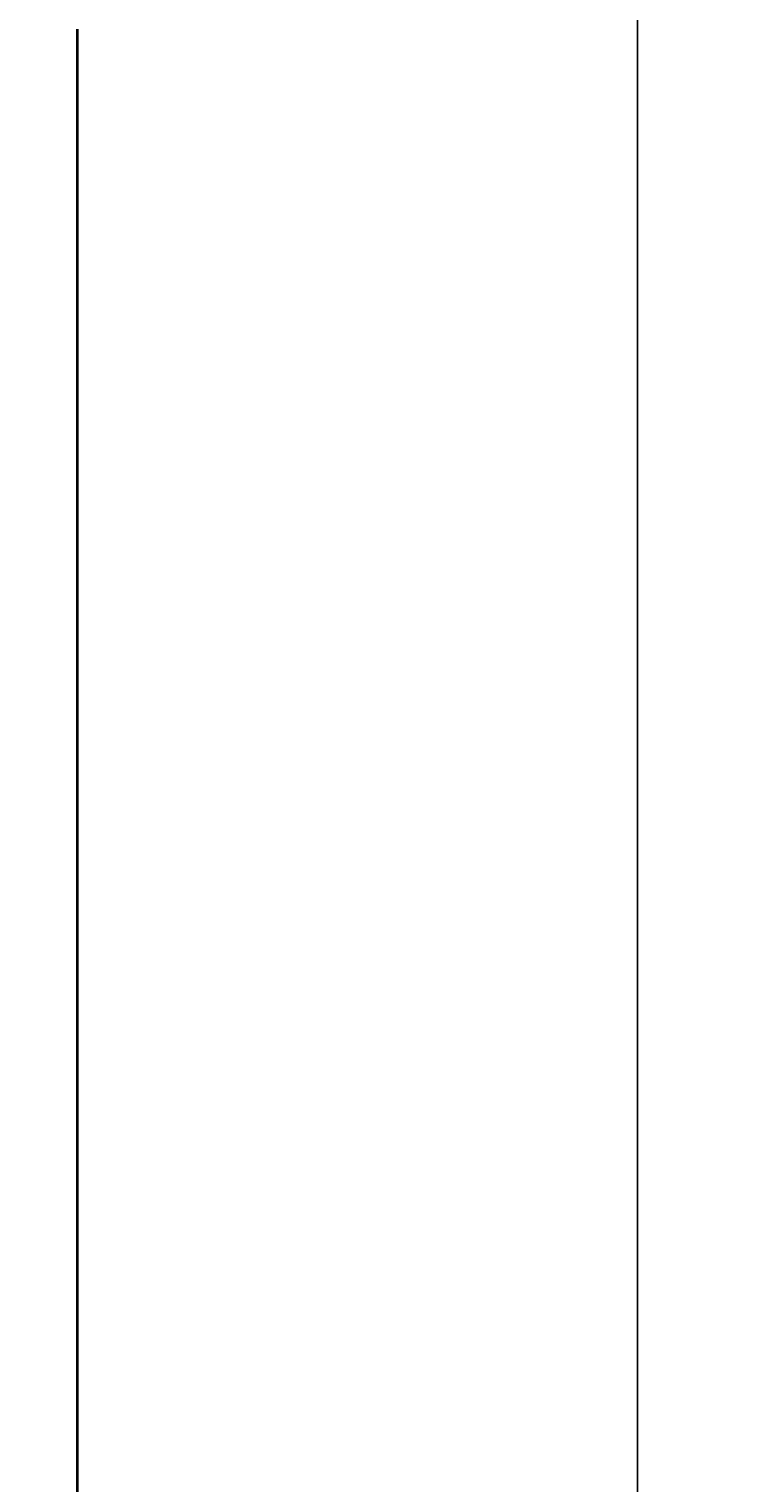
# Model space of a CAD drawing. Units: inches. Extents: x 1770 to 2988, y 1161 to 3221.
# Tile 23 of 44: x 2456 to 2524, y 2231 to 2368. Entities that reach past the tile are written whole.
import ezdxf

# ---------------------------------------------------------------- set-up
doc = ezdxf.new("R2010")
doc.units = ezdxf.units.IN
doc.layers.add('A-ANNO-DIMS', color=2, linetype='Continuous', lineweight=18)
doc.layers.add('A-WALL', color=7, linetype='Continuous', lineweight=35)
doc.styles.get("Standard").update_dxf_attribs({"font": 'arial.ttf'})
doc.dimstyles.get("Standard").update_dxf_attribs({"dimtxt": 0.18, "dimasz": 0.18, "dimexe": 0.18, "dimexo": 0.0625, "dimgap": 0.09, "dimtad": 0, "dimtih": 1, "dimtoh": 1, "dimdec": 4, "dimzin": 0, "dimdsep": 46, "dimtxsty": 'Standard', "dimcen": 0.09, "dimadec": 0, "dimazin": 0, "dimtfac": 1, "dimtdec": 4, "dimtofl": 0, "dimtmove": 0, "dimatfit": 3, "dimfxl": 1, "dimtolj": 1, "dimtzin": 0, "dimarcsym": 0})

# ---------------------------------------------------------------- blocks, each defined once
blk = doc.blocks.new('*D82')
at = {"layer": 'A-ANNO-DIMS', "color": 0, "lineweight": -2, "transparency": 16777216}
for p, q in [((2443.39, 1610.26), (2443.39, 2570.7)), ((2443.57, 2570.52), (2486.45, 2570.52)), ((2530.12, 2570.52), (2487.24, 2570.52)), ((2530.3, 1610.26), (2530.3, 2570.7))]:
    blk.add_line(p, q, dxfattribs=at)
at = {"layer": 'A-ANNO-DIMS', "color": 0, "transparency": 16777216}
for points in [[(2443.57, 2570.55), (2443.57, 2570.49), (2443.39, 2570.52)], [(2530.12, 2570.55), (2530.12, 2570.49), (2530.3, 2570.52)]]:
    blk.add_solid(points, dxfattribs=at)
at = {"layer": 'Defpoints', "color": 0, "transparency": 16777216}
for p in [(2530.3, 2570.52), (2443.39, 1610.2), (2530.3, 1610.2)]:
    blk.add_point(p, dxfattribs=at)
at = {"layer": 'A-ANNO-DIMS', "color": 0, "transparency": 16777216, "insert": (2486.85, 2570.52), "char_height": 0.18, "attachment_point": 5}
blk.add_mtext('\\A1;86.92', dxfattribs=at)
blk = doc.blocks.new('*D84')
at = {"layer": 'A-ANNO-DIMS', "color": 0, "lineweight": -2, "transparency": 16777216}
for p, q in [((2513.2, 1835.26), (2513.2, 2570.7)), ((2513.38, 2570.52), (2564.56, 2570.52)), ((2616.52, 2570.52), (2565.33, 2570.52)), ((2616.7, 1835.26), (2616.7, 2570.7))]:
    blk.add_line(p, q, dxfattribs=at)
at = {"layer": 'A-ANNO-DIMS', "color": 0, "transparency": 16777216}
for points in [[(2513.38, 2570.55), (2513.38, 2570.49), (2513.2, 2570.52)], [(2616.52, 2570.55), (2616.52, 2570.49), (2616.7, 2570.52)]]:
    blk.add_solid(points, dxfattribs=at)
at = {"layer": 'Defpoints', "color": 0, "transparency": 16777216}
for p in [(2616.7, 2570.52), (2513.2, 1835.2), (2616.7, 1835.2)]:
    blk.add_point(p, dxfattribs=at)
at = {"layer": 'A-ANNO-DIMS', "color": 0, "transparency": 16777216, "insert": (2564.95, 2570.52), "char_height": 0.18, "attachment_point": 5}
blk.add_mtext('\\A1;103.5', dxfattribs=at)

msp = doc.modelspace()

# ---------------------------------------------------------------- linework, layer by layer
at = {"layer": 'A-WALL'}
msp.add_line((2460.696, 2367.7021), (2460.696, 2175.7021), dxfattribs=at)

# ---------------------------------------------------------------- dimensions: what is measured, and where the dimension line sits
at = {"layer": 'A-ANNO-DIMS'}
for base, p1, p2, override, picture, middle in [((2530.3038, 2570.5247), (2443.3863, 1610.2021), (2530.3038, 1610.2021), {"dimdec": 2, "dimlfac": 1, "dimrnd": 0, "dimzin": 0, "dimdsep": 46, "dimlunit": 2}, '*D82', (2486.8451, 2570.5247)), ((2616.696, 2570.5247), (2513.196, 1835.2021), (2616.696, 1835.2021), {"dimdec": 1, "dimlfac": 1, "dimrnd": 0, "dimzin": 0, "dimdsep": 46, "dimlunit": 2}, '*D84', (2564.946, 2570.5247))]:
    dim = msp.add_linear_dim(base=base, p1=p1, p2=p2, dimstyle='Standard', override=override, dxfattribs=at)
    dim.commit()
    dim.dimension.update_dxf_attribs({"geometry": picture, "text_midpoint": middle})

doc.saveas('drawing.dxf')
